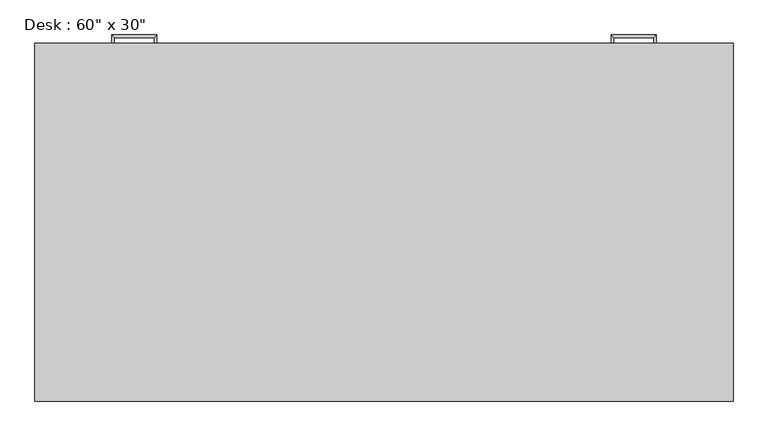
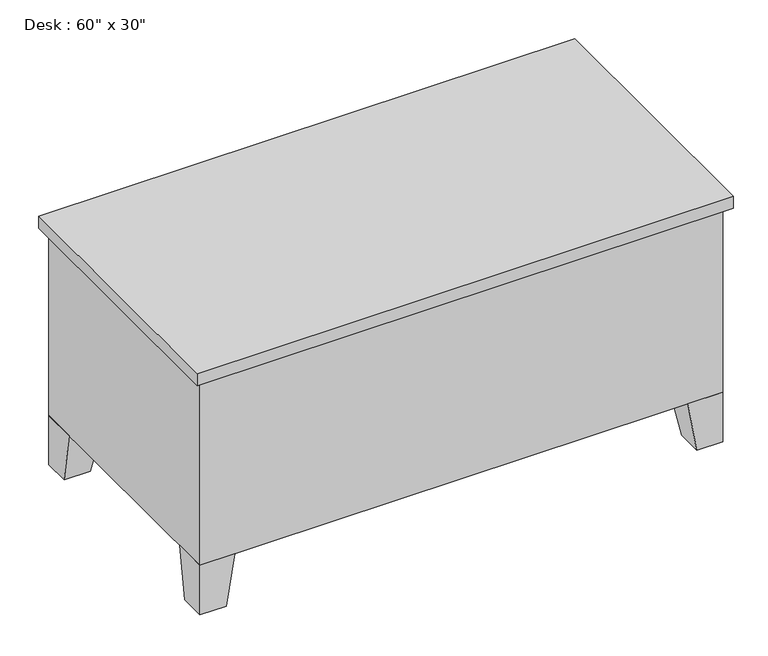
"""IFC4 building model written with IfcOpenShell, lengths in millimetres: furniture geometry."""

from ifc_helpers import new_model, si_unit, frame, origin, place, context, project, spatial, polyline, outline, extrude, faceted_brep, source, transform, mapped, element, save


def furniture_072f6425(model_context):
    return source(origin(), model_context, "Body", "SolidModel", [
        extrude(outline(polyline([(1504.95, 762.0), (1136.65, 762.0), (1136.65, 774.7), (1504.95, 774.7), (1504.95, 762.0)])), frame((0.0, 0.0, 603.25), z_axis=(0.0, 0.0, 1.0), x_axis=(1.0, 0.0, 0.0)), (0.0, 0.0, 1.0), 101.6),
        extrude(outline(polyline([(1504.95, 762.0), (1136.65, 762.0), (1136.65, 774.7), (1504.95, 774.7), (1504.95, 762.0)])), frame((0.0, 0.0, 171.45), z_axis=(0.0, 0.0, 1.0), x_axis=(1.0, 0.0, 0.0)), (0.0, 0.0, 1.0), 412.75),
        extrude(outline(polyline([(387.35, 762.0), (19.05, 762.0), (19.05, 774.7), (387.35, 774.7), (387.35, 762.0)])), frame((0.0, 0.0, 603.25), z_axis=(0.0, 0.0, 1.0), x_axis=(1.0, 0.0, 0.0)), (0.0, 0.0, 1.0), 101.6),
        extrude(outline(polyline([(387.35, 762.0), (19.05, 762.0), (19.05, 774.7), (387.35, 774.7), (387.35, 762.0)])), frame((0.0, 0.0, 171.45), z_axis=(0.0, 0.0, 1.0), x_axis=(1.0, 0.0, 0.0)), (0.0, 0.0, 1.0), 171.45),
        extrude(outline(polyline([(387.35, 762.0), (19.05, 762.0), (19.05, 774.7), (387.35, 774.7), (387.35, 762.0)])), frame((0.0, 0.0, 482.6), z_axis=(0.0, 0.0, 1.0), x_axis=(1.0, 0.0, 0.0)), (0.0, 0.0, 1.0), 101.6),
        extrude(outline(polyline([(387.35, 762.0), (19.05, 762.0), (19.05, 774.7), (387.35, 774.7), (387.35, 762.0)])), frame((0.0, 0.0, 361.95), z_axis=(0.0, 0.0, 1.0), x_axis=(1.0, 0.0, 0.0)), (0.0, 0.0, 1.0), 101.6),
        faceted_brep([(1422.4, 762.0, 152.4), (1422.4, 660.4, 152.4), (1524.0, 660.4, 152.4), (1524.0, 762.0, 152.4), (1447.8, 762.0, 0.0), (1524.0, 762.0, 0.0), (1524.0, 685.8, 0.0), (1447.8, 685.8, 0.0)], [[[0, 1, 2, 3]], [[4, 5, 6, 7]], [[4, 7, 1, 0]], [[7, 6, 2, 1]], [[6, 5, 3, 2]], [[5, 4, 0, 3]]]),
        faceted_brep([(1422.4, 0.0, 152.4), (1524.0, 0.0, 152.4), (1524.0, 101.6, 152.4), (1422.4, 101.6, 152.4), (1447.8, 0.0, 0.0), (1447.8, 76.2, 0.0), (1524.0, 76.2, 0.0), (1524.0, 0.0, 0.0)], [[[0, 1, 2, 3]], [[4, 5, 6, 7]], [[4, 7, 1, 0]], [[7, 6, 2, 1]], [[6, 5, 3, 2]], [[5, 4, 0, 3]]]),
        faceted_brep([(101.6, 0.0, 152.4), (101.6, 101.6, 152.4), (0.0, 101.6, 152.4), (0.0, 0.0, 152.4), (76.2, 0.0, 0.0), (0.0, 0.0, 0.0), (0.0, 76.2, 0.0), (76.2, 76.2, 0.0)], [[[0, 1, 2, 3]], [[4, 5, 6, 7]], [[4, 7, 1, 0]], [[7, 6, 2, 1]], [[6, 5, 3, 2]], [[5, 4, 0, 3]]]),
        faceted_brep([(101.6, 762.0, 152.4), (0.0, 762.0, 152.4), (0.0, 660.4, 152.4), (101.6, 660.4, 152.4), (76.2, 762.0, 0.0), (76.2, 685.8, 0.0), (0.0, 685.8, 0.0), (0.0, 762.0, 0.0)], [[[0, 1, 2, 3]], [[4, 5, 6, 7]], [[4, 7, 1, 0]], [[7, 6, 2, 1]], [[6, 5, 3, 2]], [[5, 4, 0, 3]]]),
        extrude(outline(polyline([(1543.05, 781.05), (1543.05, -19.05), (-19.05, -19.05), (-19.05, 781.05), (1543.05, 781.05)])), frame((0.0, 0.0, 723.9), z_axis=(0.0, 0.0, 1.0), x_axis=(1.0, 0.0, 0.0)), (0.0, 0.0, 1.0), 38.1),
        extrude(outline(polyline([(406.4, 762.0), (406.4, 50.8), (1117.6, 50.8), (1117.6, 762.0), (1524.0, 762.0), (1524.0, 0.0), (0.0, 0.0), (0.0, 762.0), (406.4, 762.0)])), frame((0.0, 0.0, 152.4), z_axis=(0.0, 0.0, 1.0), x_axis=(1.0, 0.0, 0.0)), (0.0, 0.0, 1.0), 571.5),
        faceted_brep([(1365.25, 774.7, 546.1), (1365.25, 774.7, 533.4), (1371.6, 774.7, 533.4), (1371.6, 774.7, 546.1), (1365.25, 793.75, 546.1), (1365.25, 793.75, 533.4), (1371.6, 800.1, 533.4), (1371.6, 800.1, 546.1), (1276.35, 793.75, 546.1), (1276.35, 793.75, 533.4), (1270.0, 800.1, 533.4), (1270.0, 800.1, 546.1), (1276.35, 774.7, 546.1), (1270.0, 774.7, 546.1), (1270.0, 774.7, 533.4), (1276.35, 774.7, 533.4)], [[[0, 1, 2, 3]], [[1, 0, 4, 5]], [[2, 1, 5, 6]], [[3, 2, 6, 7]], [[0, 3, 7, 4]], [[5, 4, 8, 9]], [[6, 5, 9, 10]], [[7, 6, 10, 11]], [[4, 7, 11, 8]], [[12, 13, 14, 15]], [[9, 8, 12, 15]], [[10, 9, 15, 14]], [[11, 10, 14, 13]], [[8, 11, 13, 12]]]),
        faceted_brep([(1365.25, 774.7, 666.75), (1365.25, 774.7, 654.05), (1371.6, 774.7, 654.05), (1371.6, 774.7, 666.75), (1365.25, 793.75, 666.75), (1365.25, 793.75, 654.05), (1371.6, 800.1, 654.05), (1371.6, 800.1, 666.75), (1276.35, 793.75, 666.75), (1276.35, 793.75, 654.05), (1270.0, 800.1, 654.05), (1270.0, 800.1, 666.75), (1276.35, 774.7, 666.75), (1270.0, 774.7, 666.75), (1270.0, 774.7, 654.05), (1276.35, 774.7, 654.05)], [[[0, 1, 2, 3]], [[1, 0, 4, 5]], [[2, 1, 5, 6]], [[3, 2, 6, 7]], [[0, 3, 7, 4]], [[5, 4, 8, 9]], [[6, 5, 9, 10]], [[7, 6, 10, 11]], [[4, 7, 11, 8]], [[12, 13, 14, 15]], [[9, 8, 12, 15]], [[10, 9, 15, 14]], [[11, 10, 14, 13]], [[8, 11, 13, 12]]]),
        faceted_brep([(158.75, 774.7, 304.8), (152.4, 774.7, 304.8), (152.4, 774.7, 292.1), (158.75, 774.7, 292.1), (158.75, 793.75, 304.8), (152.4, 800.1, 304.8), (152.4, 800.1, 292.1), (158.75, 793.75, 292.1), (247.65, 793.75, 304.8), (254.0, 800.1, 304.8), (254.0, 800.1, 292.1), (247.65, 793.75, 292.1), (247.65, 774.7, 304.8), (247.65, 774.7, 292.1), (254.0, 774.7, 292.1), (254.0, 774.7, 304.8)], [[[0, 1, 2, 3]], [[1, 0, 4, 5]], [[2, 1, 5, 6]], [[3, 2, 6, 7]], [[0, 3, 7, 4]], [[5, 4, 8, 9]], [[6, 5, 9, 10]], [[7, 6, 10, 11]], [[4, 7, 11, 8]], [[12, 13, 14, 15]], [[9, 8, 12, 15]], [[10, 9, 15, 14]], [[11, 10, 14, 13]], [[8, 11, 13, 12]]]),
        faceted_brep([(158.75, 774.7, 425.45), (152.4, 774.7, 425.45), (152.4, 774.7, 412.75), (158.75, 774.7, 412.75), (158.75, 793.75, 425.45), (152.4, 800.1, 425.45), (152.4, 800.1, 412.75), (158.75, 793.75, 412.75), (247.65, 793.75, 425.45), (254.0, 800.1, 425.45), (254.0, 800.1, 412.75), (247.65, 793.75, 412.75), (247.65, 774.7, 425.45), (247.65, 774.7, 412.75), (254.0, 774.7, 412.75), (254.0, 774.7, 425.45)], [[[0, 1, 2, 3]], [[1, 0, 4, 5]], [[2, 1, 5, 6]], [[3, 2, 6, 7]], [[0, 3, 7, 4]], [[5, 4, 8, 9]], [[6, 5, 9, 10]], [[7, 6, 10, 11]], [[4, 7, 11, 8]], [[12, 13, 14, 15]], [[9, 8, 12, 15]], [[10, 9, 15, 14]], [[11, 10, 14, 13]], [[8, 11, 13, 12]]]),
        faceted_brep([(158.75, 774.7, 546.1), (152.4, 774.7, 546.1), (152.4, 774.7, 533.4), (158.75, 774.7, 533.4), (158.75, 793.75, 546.1), (152.4, 800.1, 546.1), (152.4, 800.1, 533.4), (158.75, 793.75, 533.4), (247.65, 793.75, 546.1), (254.0, 800.1, 546.1), (254.0, 800.1, 533.4), (247.65, 793.75, 533.4), (247.65, 774.7, 546.1), (247.65, 774.7, 533.4), (254.0, 774.7, 533.4), (254.0, 774.7, 546.1)], [[[0, 1, 2, 3]], [[1, 0, 4, 5]], [[2, 1, 5, 6]], [[3, 2, 6, 7]], [[0, 3, 7, 4]], [[5, 4, 8, 9]], [[6, 5, 9, 10]], [[7, 6, 10, 11]], [[4, 7, 11, 8]], [[12, 13, 14, 15]], [[9, 8, 12, 15]], [[10, 9, 15, 14]], [[11, 10, 14, 13]], [[8, 11, 13, 12]]]),
        faceted_brep([(158.75, 774.7, 666.75), (152.4, 774.7, 666.75), (152.4, 774.7, 654.05), (158.75, 774.7, 654.05), (158.75, 793.75, 666.75), (152.4, 800.1, 666.75), (152.4, 800.1, 654.05), (158.75, 793.75, 654.05), (247.65, 793.75, 666.75), (254.0, 800.1, 666.75), (254.0, 800.1, 654.05), (247.65, 793.75, 654.05), (247.65, 774.7, 666.75), (247.65, 774.7, 654.05), (254.0, 774.7, 654.05), (254.0, 774.7, 666.75)], [[[0, 1, 2, 3]], [[1, 0, 4, 5]], [[2, 1, 5, 6]], [[3, 2, 6, 7]], [[0, 3, 7, 4]], [[5, 4, 8, 9]], [[6, 5, 9, 10]], [[7, 6, 10, 11]], [[4, 7, 11, 8]], [[12, 13, 14, 15]], [[9, 8, 12, 15]], [[10, 9, 15, 14]], [[11, 10, 14, 13]], [[8, 11, 13, 12]]]),
    ])


if __name__ == "__main__":
    model = new_model("IFC4")
    model_context = context("Model", 3, world=origin())
    ifc_project = project(units=[si_unit("LENGTHUNIT", "METRE", prefix="MILLI")], contexts=[model_context])
    site = spatial("IfcSite", under=ifc_project)
    building = spatial("IfcBuilding", under=site)
    placement = place(None, origin())
    furniture_shape = furniture_072f6425(model_context)
    element("IfcFurniture", 1, ObjectType="Desk : 60\" x 30\"", at=placement, inside=building, context=model_context, shape_type="MappedRepresentation", body=[
        mapped(furniture_shape, transform((0.0, 0.0, 0.0), x_axis=(1.0, 0.0, 0.0), y_axis=(0.0, 1.0, 0.0), z_axis=(0.0, 0.0, 1.0))),
    ])
    save(model, "model.ifc")

# Revit data of these elements
# Type "Desk : 60\" x 30\""
#   Assembly Code = "E2020200"
#   Depth = 2' - 6"
#   Height = 2' - 6"
#   Leg Height = 0' - 6"
#   Width = 5' - 0"
#   Body Material = Laminate, Ivory, Matte
#   Handle/Leg Material = Steel, Chrome Plated
#   Top Material = Cherry
#   Default Elevation = 0
# Element 1 (IfcFurniture, "Desk : 60\" x 30\"")
#   Materials on its faces: "Steel, Chrome Plated", "Laminate, Ivory, Matte", "Cherry"
# Materials
#   "Laminate, Ivory, Matte": class "Plastic", colour RGB 247 247 239, transparency 0, Description = "Plastic Laminate - Ivory, Matte", Cost = 0
#   "Steel, Chrome Plated": class "Metal", colour RGB 17 17 17, transparency 0, Description = "Chromiuim plated steel", Cost = 0
#   "Cherry": class "Wood", colour RGB 226 177 128, transparency 0, Description = "Prunus Serotina", Cost = 0
